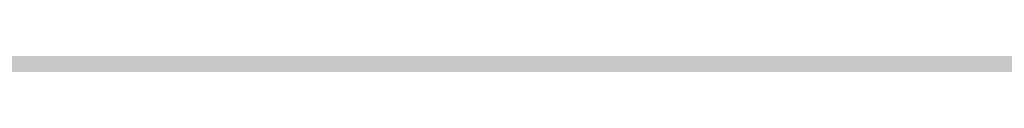
# Model space of a CAD drawing. Units: inches. Extents: x 2091 to 2899, y 967 to 2217.
# Tile 195 of 256: x 2203.18039 to 2203.25707, y 1152.24716 to 1152.24727. Entities that reach past the tile are written whole.
import ezdxf

# ---------------------------------------------------------------- set-up
doc = ezdxf.new("R2010")
doc.units = ezdxf.units.IN
doc.layers.add('A-WALL-PATT', color=141, linetype='Continuous', lineweight=13, true_color=0xadddf7)

msp = doc.modelspace()

# ---------------------------------------------------------------- hatches: boundary and pattern name
at = {"layer": 'A-WALL-PATT'}
h = msp.add_hatch(color=256, dxfattribs=at)
h.dxf.hatch_style = 1
h.paths.add_polyline_path([(2803.143603, 2050.919059), (2203.143603, 2050.919059), (2203.143603, 1090.919059), (2803.143603, 1090.919059)])
h.paths.add_polyline_path([(2635.79885, 1147.540465), (2674.524052, 1147.540465, 0.376086), (2678.529665, 1152.880202), (2678.529665, 1159.556473, 0.333335), (2674.524319, 1163.561846), (2674.524319, 1163.56185), (2674.524319, 1192.93439), (2635.805971, 1192.93439), (2597.087622, 1192.93439), (2597.087622, 1163.561846, 0.333335), (2593.082276, 1159.556473), (2593.082276, 1152.880202, 0.376086), (2597.087889, 1147.540465)], flags=0)
h.paths.add_polyline_path([(2436.010433, 1278.240778, 0.000483), (2435.952643, 1278.215027, -0.001328), (2435.935625, 1278.111693, -0.001711), (2436.11644, 1278.040758, 0.002185)], flags=0)
h.paths.add_polyline_path([(2794.143603, 1143.419059), (2794.143603, 1347.419059), (2543.370171, 1347.419059), (2543.370171, 1351.919059), (2794.143603, 1351.919059), (2794.143603, 1392.713555), (2793.947398, 1392.713555), (2793.947398, 1473.5369), (2794.143603, 1473.5369), (2794.143603, 1531.919059), (2650.143603, 1531.919059), (2650.143603, 1536.419059), (2794.143603, 1536.419059), (2794.143603, 1692.419059), (2609.375609, 1692.419059), (2609.375609, 1644.419059), (2604.875609, 1644.419059), (2604.875609, 1744.919059), (2609.375609, 1744.919059), (2609.375609, 1696.919059), (2794.143603, 1696.919059), (2794.143603, 1780.919059), (2609.643603, 1780.919059), (2493.875609, 1780.919059), (2493.875609, 1785.419059), (2609.643603, 1785.419059), (2794.143603, 1785.419059), (2794.143603, 1847.938821), (2793.951222, 1847.938821), (2793.951222, 1928.762166), (2794.143603, 1928.762166), (2794.143603, 1941.419059), (2614.143603, 1941.419059), (2614.143603, 1821.419059), (2609.643603, 1821.419059), (2609.643603, 1941.419059), (2392.143603, 1941.419059), (2392.143603, 1819.919059), (2387.643603, 1819.919059), (2387.643603, 1941.419059), (2212.143603, 1941.419059), (2212.143603, 1783.919059), (2392.143603, 1783.919059), (2392.143603, 1780.919059), (2212.143603, 1780.919059), (2212.143603, 1629.419059), (2387.643603, 1629.419059), (2387.643603, 1744.919059), (2392.143603, 1744.919059), (2392.143603, 1627.919059), (2317.143603, 1627.919059), (2317.143603, 1551.419059), (2317.143603, 1536.419059), (2459.383591, 1536.419059), (2459.383591, 1602.39648), (2463.883591, 1602.39648), (2463.883591, 1531.919059), (2456.643603, 1531.919059), (2456.643603, 1529.919059), (2452.143603, 1529.919059), (2452.143603, 1531.919059), (2312.643603, 1531.919059), (2312.643603, 1551.419059), (2306.143603, 1551.419059), (2306.143603, 1555.919059), (2308.143603, 1555.919059), (2308.143603, 1551.419059), (2312.643603, 1551.419059), (2312.643603, 1627.919059), (2212.143603, 1627.919059), (2212.143603, 1555.919059), (2270.143603, 1555.919059), (2270.143603, 1551.419059), (2212.143603, 1551.419059), (2212.143603, 1351.919059), (2272.143603, 1351.919059), (2272.143603, 1347.419059), (2212.143603, 1347.419059), (2212.143603, 1275.419059), (2308.143603, 1275.419059), (2308.143603, 1351.919059), (2452.143603, 1351.919059), (2452.143603, 1493.919059), (2456.643603, 1493.919059), (2456.643603, 1347.419059), (2312.643603, 1347.419059), (2312.643603, 1270.919059), (2212.143603, 1270.919059), (2212.143603, 1099.919059), (2281.237523, 1099.919059), (2282.871041, 1110.913803), (2282.008341, 1116.996603), (2278.557741, 1121.420403), (2268.205641, 1128.056203), (2272.087641, 1128.056203), (2273.812941, 1131.927003), (2279.420341, 1134.691903), (2285.027841, 1135.244903), (2287.615841, 1137.456803), (2288.047141, 1138.009803), (2289.341141, 1140.774703), (2291.066541, 1139.668703), (2292.360541, 1135.244903), (2295.379841, 1136.903803), (2296.242541, 1135.797903), (2297.105241, 1133.033003), (2300.124641, 1138.009803), (2303.143941, 1138.009803), (2304.437941, 1135.797903), (2303.143941, 1133.586003), (2306.594641, 1134.691903), (2307.888741, 1133.033003), (2310.908041, 1135.244903), (2313.927441, 1134.138903), (2315.62686, 1132.427102), (2308.320041, 1117.549603), (2290.203841, 1109.807903), (2288.909841, 1103.172103), (2289.272309, 1099.919059), (2434.918227, 1099.919059), (2431.593227, 1124.788059), (2429.930227, 1169.553059), (2430.927185, 1240.519694), (2435.658926, 1238.186126), (2437.135227, 1196.554059), (2438.798227, 1143.973059), (2442.678227, 1111.998059), (2446.558227, 1099.919059), (2794.143603, 1099.919059), (2794.143603, 1138.919059), (2548.032447, 1138.919059), (2548.032447, 1143.419059), (2548.032447, 1148.819059), (2546.668457, 1148.031559), (2528.685692, 1179.178622, 0.256256), (2512.032447, 1148.819059), (2512.032447, 1143.419059), (2512.032447, 1138.919059), (2507.532447, 1138.919059), (2507.532447, 1143.419059), (2507.532447, 1148.819059, 0.256256), (2490.879202, 1179.178622), (2472.896437, 1148.031559), (2471.532447, 1148.819059), (2471.532447, 1143.419059), (2467.032447, 1143.419059), (2467.032447, 1269.945786, 0.039061), (2460.909987, 1273.580059), (2467.032447, 1273.580059), (2467.032447, 1286.325364, 0.014511), (2465.216194, 1286.761905), (2467.032447, 1287.052576), (2467.032447, 1323.419059), (2471.532447, 1323.419059), (2471.532447, 1148.819059), (2489.532447, 1179.995973), (2490.896437, 1179.208473), (2490.879202, 1179.178622, -0.256256), (2507.532447, 1148.819059), (2507.532447, 1143.419059), (2512.032447, 1143.419059), (2512.032447, 1148.819059, -0.256256), (2528.685692, 1179.178622), (2528.668457, 1179.208473), (2530.032447, 1179.995973), (2548.032447, 1148.819059), (2548.032447, 1143.419059)], flags=16)
h.paths.add_polyline_path([(2607.768546, 1200.945083), (2607.768546, 1265.030625), (2597.087622, 1281.052011), (2619.784585, 1281.052011), (2627.795278, 1337.12686), (2635.79885, 1337.12686), (2643.816663, 1337.12686), (2651.827356, 1281.052011), (2674.524319, 1281.052011), (2663.843395, 1265.030625), (2663.843395, 1200.945083), (2635.805971, 1200.945083)], flags=0)
edge = h.paths.add_edge_path(flags=0)
edge.add_ellipse((13303.896215, 1272.998725), major_axis=(-10595.31304, 0.000001), ratio=0.842303870086, start_angle=0.6282372191, end_angle=0.6465540999, ccw=False)
edge.add_ellipse((2711.70045, 1156.852678), major_axis=(2.219769, 0), ratio=0.84230387, start_angle=111.535244, end_angle=180.628237, ccw=False)
edge.add_ellipse((13303.156292, 1272.998725), major_axis=(-10593.026306, 0), ratio=0.842303869544, start_angle=0.5282714718, end_angle=0.6465540971, ccw=False)
edge.add_line((2710.764596, 1175.333295), (2710.129986, 1175.333295))
edge.add_ellipse((2710.129986, 1176.579775), major_axis=(1.479846, 0), ratio=0.84230387, start_angle=180, end_angle=270, ccw=False)
edge.add_line((2708.65014, 1176.579775), (2708.65014, 1200.782914))
edge.add_ellipse((2710.129986, 1200.782914), major_axis=(1.479846, 0), ratio=0.84230387, start_angle=90, end_angle=180, ccw=False)
edge.add_line((2710.129986, 1202.029394), (2710.465075, 1202.029394))
edge.add_ellipse((13303.156292, 1272.998725), major_axis=(-10593.026306, 0), ratio=0.842303869544, start_angle=-0.0902290886, end_angle=0.3838667788, ccw=False)
edge.add_ellipse((2710.129986, 1290.927031), major_axis=(-1.479846, 0), ratio=0.84230387, start_angle=0, end_angle=90, ccw=False)
edge.add_line((2708.65014, 1290.927031), (2708.65014, 1315.13017))
edge.add_ellipse((2710.129986, 1315.13017), major_axis=(-1.479846, 0), ratio=0.84230387, start_angle=-90, end_angle=0, ccw=False)
edge.add_line((2710.129986, 1316.37665), (2710.706314, 1316.37665))
edge.add_ellipse((3238.40172, 1296.289566), major_axis=(528.234, 0), ratio=0.8423038695, start_angle=176.34957241, end_angle=177.82004969, ccw=False)
edge.add_ellipse((2775.063043, 1071.450696), major_axis=(313.307761, 0), ratio=0.8423038695, start_angle=102.12596555, end_angle=103.78052899, ccw=False)
edge.add_ellipse((2775.063043, 1078.305698), major_axis=(-305.302891, 0), ratio=0.8423038695, start_angle=-79.790461, end_angle=-77.55537271, ccw=False)
edge.add_ellipse((2695.141767, 1541.975383), major_axis=(-250.960216, 0), ratio=0.8423038695, start_angle=99.25656601, end_angle=102.55493264)
edge.add_line((2741.410326, 1334.214255), (2747.132545, 1337.378477))
edge.add_ellipse((2747.538616, 1336.857478), major_axis=(-0.739923, 0), ratio=0.8423039, start_angle=270, end_angle=307.93313, ccw=False)
edge.add_ellipse((2747.538616, 1336.857478), major_axis=(-0.739923, 0), ratio=0.8423039, start_angle=232.06687, end_angle=270, ccw=False)
edge.add_line((2747.944687, 1337.378477), (2753.666906, 1334.214255))
edge.add_ellipse((2799.935466, 1541.975383), major_axis=(250.960216, 0), ratio=0.8423038695, start_angle=257.44506736, end_angle=260.74343399)
edge.add_ellipse((2720.014189, 1078.305698), major_axis=(305.302891, 0), ratio=0.8423038695, start_angle=77.55537271, end_angle=79.790461, ccw=False)
edge.add_ellipse((2720.014189, 1071.450696), major_axis=(-313.307761, 0), ratio=0.8423038695, start_angle=256.21947101, end_angle=257.87403445, ccw=False)
edge.add_ellipse((2256.675512, 1296.289566), major_axis=(-528.234, 0), ratio=0.8423038695, start_angle=182.17995031, end_angle=183.65042759, ccw=False)
edge.add_line((2784.370918, 1316.37665), (2784.947247, 1316.37665))
edge.add_ellipse((2784.947247, 1315.13017), major_axis=(1.479846, 0), ratio=0.84230387, start_angle=0, end_angle=90, ccw=False)
edge.add_line((2786.427093, 1315.13017), (2786.427093, 1290.927031))
edge.add_ellipse((2784.947247, 1290.927031), major_axis=(1.479846, 0), ratio=0.84230387, start_angle=270, end_angle=360, ccw=False)
edge.add_ellipse((-7808.07906, 1272.998725), major_axis=(10593.026306, 0), ratio=0.842303869544, start_angle=-0.3838667788, end_angle=0.0902290886, ccw=False)
edge.add_line((2784.612157, 1202.029394), (2784.947247, 1202.029394))
edge.add_ellipse((2784.947247, 1200.782914), major_axis=(1.479846, 0), ratio=0.84230387, start_angle=0, end_angle=90, ccw=False)
edge.add_line((2786.427093, 1200.782914), (2786.427093, 1176.579775))
edge.add_ellipse((2784.947247, 1176.579775), major_axis=(-1.479846, 0), ratio=0.84230387, start_angle=90, end_angle=180, ccw=False)
edge.add_line((2784.947247, 1175.333295), (2784.312636, 1175.333295))
edge.add_ellipse((-7808.07906, 1272.998725), major_axis=(10593.026306, 0), ratio=0.842303869544, start_angle=-0.6186431963, end_angle=-0.5282714718, ccw=False)
edge.add_ellipse((2783.376783, 1156.852678), major_axis=(-2.219769, 0), ratio=0.84230387, start_angle=179.371763, end_angle=248.464757, ccw=False)
edge.add_ellipse((-7808.818983, 1272.998725), major_axis=(-10595.31304, 0.000004), ratio=0.842303865762, start_angle=179.3534459226, end_angle=179.3717628034, ccw=False)
edge.add_ellipse((2780.297303, 1153.500793), major_axis=(-5.246426, 0), ratio=0.84230387, start_angle=90, end_angle=179.353446, ccw=False)
edge.add_line((2780.297303, 1149.081708), (2714.77993, 1149.081708))
edge.add_ellipse((2714.77993, 1153.500793), major_axis=(5.246426, 0), ratio=0.84230387, start_angle=180.646554, end_angle=270, ccw=False)
edge = h.paths.add_edge_path(flags=0)
edge.add_line((2718.187367, 1151.007833), (2718.187367, 1170.472364))
edge.add_ellipse((2721.14706, 1170.472364), major_axis=(-2.959692, 0), ratio=0.84230387, start_angle=-90, end_angle=0, ccw=False)
edge.add_line((2721.14706, 1172.965324), (2773.930173, 1172.965324))
edge.add_ellipse((2773.930173, 1170.472364), major_axis=(-2.959692, 0), ratio=0.84230387, start_angle=180, end_angle=270, ccw=False)
edge.add_line((2776.889865, 1170.472364), (2776.889865, 1151.007833))
edge.add_line((2776.889865, 1151.007833), (2718.187367, 1151.007833))
edge = h.paths.add_edge_path(flags=0)
edge.add_line((2718.187367, 1180.23415), (2718.187367, 1199.057834))
edge.add_ellipse((2747.538616, 1320.39864), major_axis=(147.017924, 0), ratio=0.8423038695, start_angle=256.40186531, end_angle=283.59813469)
edge.add_line((2776.889865, 1199.057834), (2776.889865, 1180.23415))
edge.add_ellipse((2747.538616, 1301.574956), major_axis=(147.017924, 0), ratio=0.8423038695, start_angle=256.40186531, end_angle=283.59813469, ccw=False)
edge = h.paths.add_edge_path(flags=0)
edge.add_ellipse((13303.156292, 1272.998725), major_axis=(-10591.54646, 0), ratio=0.842303869555, start_angle=0.0555943135, end_angle=0.3777641939, ccw=False)
edge.add_line((2711.616859, 1262.72171), (2715.667408, 1249.495396))
edge.add_ellipse((6413.891963, 1241.691919), major_axis=(-3698.236159, 0), ratio=0.84230386955, start_angle=-0.120897369, end_angle=0.364076349)
edge.add_line((2715.761038, 1218.192455), (2711.934307, 1203.167361))
edge = h.paths.add_edge_path(flags=0)
edge.add_line((2718.187367, 1251.074566), (2716.002485, 1267.450435))
edge.add_ellipse((2742.151175, 1202.18954), major_axis=(81.772585, 0), ratio=0.84230387, start_angle=94.27742096, end_angle=111.8349538, ccw=False)
edge.add_line((2737.009748, 1270.930626), (2758.067484, 1270.930626))
edge.add_ellipse((2752.926058, 1202.18954), major_axis=(81.772585, 0), ratio=0.84230387, start_angle=68.1650462, end_angle=85.72257904, ccw=False)
edge.add_line((2779.074747, 1267.450435), (2776.889865, 1251.074566))
edge.add_ellipse((2750.338059, 1187.885356), major_axis=(79.579664, 0), ratio=0.84230387, start_angle=67.20808512, end_angle=85.1299304)
edge.add_line((2756.034656, 1254.743656), (2739.042576, 1254.743656))
edge.add_ellipse((2744.739174, 1187.885356), major_axis=(79.579664, 0), ratio=0.84230387, start_angle=94.8700696, end_angle=112.79191488)
edge = h.paths.add_edge_path(flags=0)
edge.add_line((2783.142926, 1203.167361), (2779.316194, 1218.192455))
edge.add_ellipse((-918.81473, 1241.691919), major_axis=(3698.236159, 0), ratio=0.84230386955, start_angle=-0.364076349, end_angle=0.120897369)
edge.add_line((2779.409825, 1249.495396), (2783.460373, 1262.72171))
edge.add_ellipse((-7808.07906, 1272.998725), major_axis=(-10591.54646, 0), ratio=0.84230386954, start_angle=179.6222358061, end_angle=179.9444056865, ccw=False)
edge = h.paths.add_edge_path(flags=0)
edge.add_ellipse((2734.200892, 1286.69044), major_axis=(-0.356609, 6.340078), ratio=0.60383358, start_angle=89.0020143, end_angle=253.657408, ccw=False)
edge.add_line((2730.369001, 1286.541806), (2730.369001, 1301.35198))
edge.add_line((2730.369001, 1301.35198), (2735.913311, 1305.214803))
edge.add_ellipse((2736.384917, 1304.734561), major_axis=(0.739923, 0), ratio=0.8423039, start_angle=90, end_angle=134.480211, ccw=False)
edge.add_line((2736.384917, 1305.357801), (2738.032783, 1305.357801))
edge.add_line((2738.032783, 1305.357801), (2738.032783, 1307.707927))
edge.add_ellipse((2794.201642, 1307.707927), major_axis=(56.168859, 0), ratio=0.84230387, start_angle=150.5614304, end_angle=180, ccw=False)
edge.add_ellipse((2700.875591, 1307.707927), major_axis=(-56.168859, 0), ratio=0.84230387, start_angle=180, end_angle=209.4385696, ccw=False)
edge.add_line((2757.04445, 1307.707927), (2757.04445, 1305.357801))
edge.add_line((2757.04445, 1305.357801), (2758.692316, 1305.357801))
edge.add_ellipse((2758.692316, 1304.734561), major_axis=(-0.739923, 0), ratio=0.8423039, start_angle=225.519789, end_angle=270, ccw=False)
edge.add_line((2759.163922, 1305.214803), (2764.708231, 1301.35198))
edge.add_line((2764.708231, 1301.35198), (2764.708231, 1286.541806))
edge.add_ellipse((2760.87634, 1286.69044), major_axis=(0.356609, 6.340078), ratio=0.60383358, start_angle=106.342592, end_angle=270.9979857, ccw=False)
edge.add_line((2757.04445, 1285.79709), (2757.04445, 1307.707927))
edge.add_ellipse((2700.875591, 1307.707927), major_axis=(-56.168859, 0), ratio=0.84230387, start_angle=180, end_angle=209.4385696)
edge.add_ellipse((2794.201642, 1307.707927), major_axis=(56.168859, 0), ratio=0.84230387, start_angle=150.5614304, end_angle=180)
edge.add_line((2738.032783, 1307.707927), (2738.032783, 1285.79709))
h.paths.add_polyline_path([(2417.812273, 1104.449704), (2413.492273, 1102.529704), (2410.612273, 1103.969704), (2409.172273, 1106.369704), (2407.252273, 1107.329704), (2406.292273, 1109.729704), (2405.332273, 1114.049704), (2405.332273, 1117.889704), (2406.292273, 1120.129704), (2407.252273, 1119.809704), (2408.848322, 1118.327658), (2410.173945, 1119.42417), (2410.211273, 1120.405704), (2411.040731, 1121.419054), (2410.699273, 1119.858704), (2410.173945, 1119.42417), (2410.088452, 1117.176109), (2411.132836, 1116.206324), (2413.972273, 1119.329704), (2416.852273, 1120.769704), (2416.869721, 1120.798784), (2417.035071, 1119.405116), (2417.896213, 1118.143384), (2418.292273, 1118.369704), (2419.544447, 1120.039269), (2419.360915, 1118.387487), (2419.032108, 1119.356151), (2418.398939, 1118.511926), (2419.252273, 1114.529704), (2418.794091, 1107.198795)], flags=0)
h.paths.add_polyline_path([(2508.870171, 1347.419059), (2508.370171, 1347.419059), (2508.370171, 1351.919059), (2508.870171, 1351.919059)], flags=0)
h.paths.add_polyline_path([(2473.370171, 1347.419059), (2472.370171, 1347.419059), (2467.870171, 1347.419059), (2467.870171, 1455.419059), (2472.370171, 1455.419059), (2472.370171, 1352.419059), (2473.370171, 1352.419059)], flags=0)
h.paths.add_polyline_path([(2352.106244, 1217.446197), (2349.226244, 1218.886197), (2347.786244, 1221.286197), (2345.866244, 1222.246197), (2344.906244, 1224.646197), (2343.946244, 1228.966197), (2343.946244, 1232.806197), (2344.906244, 1235.046197), (2345.866244, 1234.726197), (2347.462293, 1233.244152), (2348.787916, 1234.340663), (2348.825244, 1235.322197), (2349.654702, 1236.335547), (2349.313244, 1234.775197), (2348.787916, 1234.340663), (2348.702423, 1232.092603), (2349.746807, 1231.122817), (2352.586244, 1234.246197), (2355.466244, 1235.686197), (2355.483692, 1235.715277), (2355.649043, 1234.321609), (2356.510185, 1233.059877), (2356.906244, 1233.286197), (2358.158418, 1234.955762), (2357.974887, 1233.30398), (2357.646079, 1234.272644), (2357.012911, 1233.428419), (2357.866244, 1229.446197), (2357.408062, 1222.115288), (2356.426244, 1219.366197)], flags=0)
h.paths.add_polyline_path([(2348.2968, 1112.22442), (2347.0138, 1112.31042), (2345.5298, 1114.12742), (2345.7318, 1115.85842), (2346.8118, 1116.98242), (2346.8118, 1114.64642), (2345.8668, 1114.21442), (2346.8798, 1114.30042)], flags=0)
h.paths.add_polyline_path([(2347.0138, 1110.92642), (2346.2718, 1110.49342), (2346.6098, 1111.18642)], flags=0)
h.paths.add_polyline_path([(2345.8668, 1118.19442), (2345.5298, 1117.32942), (2343.7078, 1118.02142), (2344.3828, 1118.62642)], flags=0)
h.paths.add_polyline_path([(2346.6768, 1109.28242), (2346.0698, 1108.07142), (2345.8668, 1110.06142)], flags=0)
h.paths.add_polyline_path([(2345.0568, 1119.75142), (2343.6398, 1119.75142), (2343.9778, 1121.13542)], flags=0)
h.paths.add_polyline_path([(2345.2598, 1116.55042), (2345.1248, 1115.85842), (2344.9218, 1115.68542), (2344.7198, 1116.37742)], flags=0)
h.paths.add_polyline_path([(2345.6648, 1112.31042), (2345.4618, 1111.53242), (2344.0448, 1111.96442), (2344.6518, 1112.57042)], flags=0)
h.paths.add_polyline_path([(2345.1918, 1113.34942), (2344.4498, 1113.86842), (2344.7198, 1114.38742)], flags=0)
h.paths.add_polyline_path([(2344.6518, 1116.80942), (2344.1798, 1115.68542), (2344.6518, 1115.33942), (2343.9098, 1114.90642), (2343.0328, 1115.94442), (2343.6398, 1116.46342)], flags=0)
h.paths.add_polyline_path([(2345.8668, 1106.68642), (2344.9898, 1105.56242), (2344.5168, 1106.60042)], flags=0)
h.paths.add_polyline_path([(2344.8548, 1110.06142), (2344.5168, 1109.28242), (2344.1128, 1109.71542)], flags=0)
h.paths.add_polyline_path([(2344.0448, 1113.52242), (2343.4378, 1113.08942), (2342.7628, 1113.95442)], flags=0)
h.paths.add_polyline_path([(2344.3148, 1111.01242), (2342.9648, 1110.32042), (2342.9648, 1111.09942)], flags=0)
h.paths.add_polyline_path([(2345.1248, 1104.69742), (2344.5848, 1103.74542), (2344.4498, 1104.26442)], flags=0)
h.paths.add_polyline_path([(2342.8298, 1121.22242), (2341.7498, 1120.53042), (2340.5358, 1121.04942), (2340.1308, 1121.82842), (2340.6708, 1122.95242), (2341.1428, 1121.82842), (2341.6148, 1122.00142)], flags=0)
h.paths.add_polyline_path([(2342.9648, 1119.75142), (2343.0328, 1118.45342), (2342.0878, 1118.02142), (2342.0198, 1119.49142)], flags=0)
h.paths.add_polyline_path([(2342.6948, 1116.89642), (2341.9528, 1116.63642), (2342.0198, 1117.32942)], flags=0)
h.paths.add_polyline_path([(2343.0328, 1112.22442), (2342.0198, 1111.79142), (2341.5478, 1112.22442), (2342.3578, 1113.34942)], flags=0)
h.paths.add_polyline_path([(2343.7748, 1104.43742), (2342.6278, 1102.88042), (2342.6948, 1104.61042), (2343.4378, 1105.12942)], flags=0)
h.paths.add_polyline_path([(2342.0198, 1115.07942), (2340.8058, 1115.51242), (2340.9408, 1116.37742)], flags=0)
h.paths.add_polyline_path([(2341.4808, 1120.09742), (2341.4808, 1119.40542), (2341.0758, 1119.57842), (2341.1428, 1120.09742)], flags=0)
h.paths.add_polyline_path([(2341.8178, 1114.47342), (2340.9408, 1113.08942), (2340.8058, 1114.56042)], flags=0)
h.paths.add_polyline_path([(2341.1428, 1118.54042), (2340.9408, 1116.98242), (2339.0508, 1117.67542), (2339.0508, 1118.62642)], flags=0)
h.paths.add_polyline_path([(2342.6948, 1101.66842), (2341.9528, 1101.84142), (2342.5598, 1102.36142)], flags=0)
h.paths.add_polyline_path([(2340.3328, 1119.66542), (2338.4438, 1119.57842), (2337.9038, 1120.35742), (2339.6578, 1120.61642)], flags=0)
h.paths.add_polyline_path([(2340.3328, 1115.33942), (2340.0628, 1113.69542), (2339.3878, 1115.33942)], flags=0)
h.paths.add_polyline_path([(2341.8178, 1103.83142), (2341.5478, 1102.88042), (2341.1428, 1103.65842)], flags=0)
h.paths.add_polyline_path([(2339.0508, 1122.86642), (2337.2958, 1121.82842), (2337.0938, 1123.12542), (2337.7688, 1123.81842)], flags=0)
h.paths.add_polyline_path([(2339.1178, 1121.74142), (2338.8478, 1121.22242), (2338.1738, 1121.04942), (2338.3758, 1121.56842)], flags=0)
h.paths.add_polyline_path([(2339.1858, 1119.31942), (2338.6458, 1118.71342), (2338.2408, 1118.10742), (2338.2408, 1118.88642)], flags=0)
h.paths.add_polyline_path([(2341.1428, 1101.92842), (2340.6028, 1101.23642), (2340.0628, 1101.84142), (2340.6028, 1102.36142)], flags=0)
h.paths.add_polyline_path([(2337.6338, 1117.76142), (2336.6208, 1118.28042), (2337.2958, 1118.97242)], flags=0)
h.paths.add_polyline_path([(2336.8238, 1119.57842), (2334.7988, 1118.97242), (2335.2038, 1120.35742), (2336.5538, 1120.87642)], flags=0)
h.paths.add_polyline_path([(2339.1178, 1100.45742), (2337.3638, 1100.54342), (2336.7558, 1101.23642)], flags=0)
h.paths.add_polyline_path([(2336.3508, 1122.43342), (2336.0138, 1121.91442), (2334.9338, 1122.43342), (2334.5288, 1123.47142), (2335.7438, 1122.77942)], flags=0)
h.paths.add_polyline_path([(2334.7318, 1120.87642), (2334.2588, 1120.35742), (2334.0568, 1120.78942), (2334.5968, 1121.30842)], flags=0)
h.paths.add_polyline_path([(2334.4618, 1122.17442), (2332.5718, 1121.30842), (2331.3568, 1122.17442), (2332.0998, 1122.86642)], flags=0)
h.paths.add_polyline_path([(2334.2588, 1118.54042), (2333.3818, 1118.45342), (2333.6518, 1119.31942)], flags=0)
h.paths.add_polyline_path([(2335.5418, 1102.27442), (2334.1918, 1102.62042), (2335.2718, 1103.31242)], flags=0)
h.paths.add_polyline_path([(2332.7068, 1119.66542), (2331.6948, 1120.44342), (2332.5048, 1120.78942)], flags=0)
h.paths.add_polyline_path([(2334.7318, 1101.14942), (2333.5168, 1101.58242), (2333.9888, 1101.75542)], flags=0)
h.paths.add_polyline_path([(2332.6398, 1116.63642), (2331.0868, 1116.29042), (2331.9648, 1118.19442)], flags=0)
h.paths.add_polyline_path([(2330.7498, 1121.56842), (2330.2768, 1120.27042), (2328.5228, 1119.31942), (2328.9948, 1121.04942)], flags=0)
h.paths.add_polyline_path([(2330.7498, 1118.62642), (2330.0078, 1117.50242), (2329.8728, 1118.02142)], flags=0)
h.paths.add_polyline_path([(2332.0998, 1102.36142), (2330.5468, 1102.01442), (2331.6948, 1102.96642)], flags=0)
h.paths.add_polyline_path([(2329.5348, 1113.60842), (2329.0628, 1112.31042), (2328.5898, 1113.34942)], flags=0)
h.paths.add_polyline_path([(2328.3878, 1117.84842), (2327.5098, 1116.55042), (2327.1728, 1117.76142)], flags=0)
h.paths.add_polyline_path([(2329.7378, 1106.51342), (2329.5348, 1105.30242), (2328.2528, 1106.08142)], flags=0)
h.paths.add_polyline_path([(2328.6578, 1114.38742), (2328.0498, 1114.12742), (2328.3198, 1114.90642)], flags=0)
h.paths.add_polyline_path([(2328.3198, 1112.22442), (2327.1058, 1112.13742), (2326.7008, 1112.65642)], flags=0)
h.paths.add_polyline_path([(2326.9028, 1115.25242), (2326.7008, 1114.12742), (2325.2158, 1113.60842), (2326.0928, 1115.33942)], flags=0)
h.paths.add_polyline_path([(2326.6328, 1108.33042), (2326.0928, 1107.37942), (2325.8908, 1108.50342), (2326.4978, 1109.10942)], flags=0)
h.paths.add_polyline_path([(2615.143603, 1531.919059), (2609.643603, 1531.919059), (2609.643603, 1620.419059), (2614.143603, 1620.419059), (2614.143603, 1536.419059), (2615.143603, 1536.419059)], flags=0)
h.paths.add_polyline_path([(2545.143603, 1563.419059), (2464.143603, 1563.419059), (2464.143603, 1632.419059), (2509.143603, 1632.419059), (2509.143603, 1627.919059), (2509.143603, 1603.919059), (2468.643603, 1603.919059), (2468.643603, 1567.919059), (2540.643603, 1567.919059), (2540.643603, 1591.919059), (2545.143603, 1591.919059)], flags=0)
h.paths.add_polyline_path([(2388.969048, 1549.985735), (2357.434181, 1549.985735), (2357.434181, 1623.360778), (2399.362777, 1623.360778), (2435.689465, 1623.360778), (2435.592547, 1602.559273), (2435.592547, 1602.39648), (2388.969048, 1602.39648)], flags=0)
h.paths.add_polyline_path([(2388.880628, 1555.809151), (2374.904429, 1555.809151), (2374.904429, 1600.571564), (2374.904429, 1615.457645), (2406.350877, 1615.457645), (2406.350877, 1618.939431), (2412.174293, 1615.457645), (2406.350877, 1611.97586), (2406.350877, 1615.457645), (2388.880628, 1615.457645)], flags=0)
h.paths.add_polyline_path([(2568.875609, 1644.419059), (2453.375609, 1644.419059), (2453.375609, 1785.419059), (2457.875609, 1785.419059), (2457.875609, 1648.919059), (2568.875609, 1648.919059)], flags=0)
h.paths.add_polyline_path([(2212.143603, 1945.919059), (2212.143603, 2041.919059), (2794.143603, 2041.919059), (2794.143603, 1945.919059)], flags=16)
h.paths.add_polyline_path([(2271.082728, 1964.317238), (2776.852968, 1964.317238), (2776.852968, 2037.169623), (2271.082728, 2037.169623)], flags=8)
h.paths.add_polyline_path([(2380.649285, 1536.824144), (2461.040809, 1536.824144), (2461.040809, 1554.652587), (2380.649285, 1554.652587)], flags=8)
h.paths.add_polyline_path([(2240.755709, 1609.725451), (2309.185829, 1609.725451), (2309.185829, 1617.698204), (2240.755709, 1617.698204)], flags=8)
h.paths.add_polyline_path([(2212.677255, 1313.504102), (2282.59152, 1313.504102), (2282.59152, 1322.745239), (2212.677255, 1322.745239)], flags=8)
h.paths.add_polyline_path([(2457.111976, 1114.778574), (2558.481581, 1114.778574), (2558.481581, 1142.219682), (2457.111976, 1142.219682)], flags=8)
h.paths.add_polyline_path([(2473.442337, 1273.010067), (2604.641226, 1273.010067), (2604.641226, 1318.346935), (2473.442337, 1318.346935)], flags=8)
h.paths.add_polyline_path([(2638.876302, 1626.977432), (2684.250367, 1627.976738), (2684.038483, 1637.597494), (2638.664417, 1636.598188)], flags=8)
h.paths.add_polyline_path([(2537.590554, 1453.793447), (2628.389547, 1453.793447), (2628.389547, 1475.344811), (2537.590554, 1475.344811)], flags=8)
h.paths.add_polyline_path([(2504.137638, 1714.632397), (2554.647187, 1714.632397), (2554.647187, 1730.237712), (2504.137638, 1730.237712)], flags=8)
h.paths.add_polyline_path([(2487.501181, 1575.651872), (2535.097121, 1575.651872), (2535.097121, 1598.377646), (2487.501181, 1598.377646)], flags=8)
h.paths.add_polyline_path([(2709.0994, 1735.710278), (2740.016601, 1735.710278), (2740.016601, 1749.937641), (2709.0994, 1749.937641)], flags=8)
h.paths.add_polyline_path([(2442.438424, 1792.171657), (2564.728835, 1792.171657), (2564.728835, 1842.000163), (2442.438424, 1842.000163)], flags=8)
h.paths.add_polyline_path([(2655.815801, 1809.644076), (2789.520142, 1806.693796), (2790.084977, 1832.291638), (2656.380635, 1835.241918)], flags=8)
h.paths.add_polyline_path([(2234.842697, 1797.720143), (2368.592851, 1794.768852), (2369.160718, 1820.504132), (2235.410564, 1823.455423)], flags=8)
h.paths.add_polyline_path([(2245.138466, 1644.006335), (2398.427733, 1640.6239), (2398.994842, 1666.32482), (2245.705575, 1669.707255)], flags=8)
h.paths.add_polyline_path([(2306.142847, 1431.168519), (2413.768314, 1428.793687), (2414.333148, 1454.391529), (2306.707682, 1456.76636)], flags=8)
h.paths.add_polyline_path([(2306.834582, 1458.233145), (2393.380484, 1456.323449), (2393.932808, 1481.354358), (2307.386907, 1483.264054)], flags=8)

doc.saveas('drawing.dxf')
